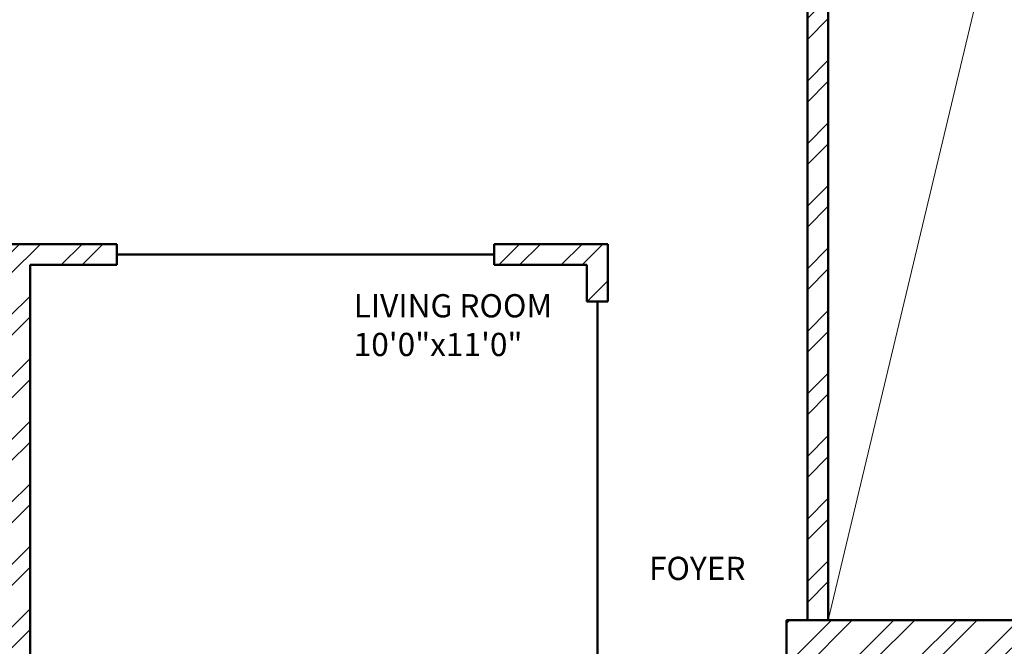
# Model space of a CAD drawing. Units: inches. Extents: x 1901 to 2863, y 888 to 2433.
# Tile 53 of 91: x 2169 to 2381, y 1867 to 2002. Entities that reach past the tile are written whole.
import ezdxf

# ---------------------------------------------------------------- set-up
doc = ezdxf.new("R2010")
doc.units = ezdxf.units.IN
for name, color, linetype, lineweight in [('A-ANNO-SYMB', 8, 'Continuous', 13), ('A-AREA-IDEN', 7, 'Continuous', 18), ('A-WALL', 7, 'Continuous', 50), ('A-WALL-PATT', 8, 'Continuous', 13)]:
    doc.layers.add(name, color=color, linetype=linetype, lineweight=lineweight)
doc.styles.get("Standard").update_dxf_attribs({"font": 'arial.ttf'})

msp = doc.modelspace()

# ---------------------------------------------------------------- hatches: boundary and pattern name
at = {"layer": 'A-WALL-PATT'}
h = msp.add_hatch(dxfattribs=at)
h.set_pattern_fill('ANSI32', color=256)
h.paths.add_polyline_path([(2192.5, 2274.13), (2141.26, 2274.13), (2141.26, 2269.63), (2192.5, 2269.63)])
h.paths.add_polyline_path([(2259.93, 2274.13), (2216.5, 2274.13), (2216.5, 2269.63), (2255.43, 2269.63), (2255.43, 2214.63), (2250.81, 2214.63), (2250.81, 2210.13), (2259.93, 2210.13), (2259.93, 2215.13), (2271.76, 2215.13), (2271.76, 2217.38), (2271.76, 2219.63), (2259.93, 2219.63)])
h.paths.add_polyline_path([(2171.43, 2269.63), (2166.93, 2269.63), (2166.93, 2219.63), (2121.24, 2219.63), (2121.24, 2215.13), (2166.93, 2215.13), (2166.93, 2083.13), (2161.81, 2083.13), (2161.81, 2078.63), (2171.43, 2078.63), (2177, 2078.63), (2177, 2080.88), (2177, 2083.13), (2171.43, 2083.13), (2171.43, 2210.13), (2230.91, 2210.13), (2230.91, 2212.38), (2230.91, 2214.63), (2171.43, 2214.63)])
h.paths.add_polyline_path([(2117.26, 2274.13), (2089.43, 2274.13), (2089.43, 2219.63), (2081.14, 2219.63), (2081.14, 2215.13), (2089.43, 2215.13), (2098, 2215.13), (2098, 2217.38), (2098, 2219.63), (2093.93, 2219.63), (2093.93, 2269.63), (2117.26, 2269.63), (2117.26, 2271.88)])
h.paths.add_polyline_path([(2343.43, 2219.63), (2329.29, 2219.63), (2329.29, 2215.13), (2338.93, 2215.13), (2338.93, 2184.74), (2343.43, 2184.74)])
h.paths.add_polyline_path([(2338.93, 2083.13), (2329.29, 2083.13), (2208.97, 2083.13), (2208.97, 2078.63), (2338.93, 2078.63)])
h.paths.add_polyline_path([(2343.43, 2136.74), (2338.93, 2136.74), (2338.93, 1872.63), (2343.43, 1872.63)])
h.paths.add_polyline_path([(2343.43, 1863.63), (2397.68, 1863.63), (2397.68, 1821.63), (2384.14, 1821.63), (2384.14, 1812.63), (2418.33, 1812.63), (2418.33, 1817.13), (2418.33, 1821.63), (2406.68, 1821.63), (2406.68, 1863.63), (2459.5, 1863.63), (2459.5, 1821.63), (2447.14, 1821.63), (2447.14, 1812.63), (2459.5, 1812.63), (2468.5, 1812.63), (2468.5, 1872.63), (2394.43, 1872.63), (2334.43, 1872.63), (2334.43, 1812.63), (2343.43, 1812.63), (2353.25, 1812.63), (2353.25, 1821.63), (2343.43, 1821.63)])
h.paths.add_polyline_path([(2510.01, 1872.63), (2468.5, 1872.63), (2468.5, 1868.13), (2510.01, 1868.13)])
h.paths.add_polyline_path([(2514.01, 1817.13), (2468.5, 1817.13), (2468.5, 1812.63), (2482.11, 1812.63), (2482.11, 1800.61), (2486.61, 1800.61), (2486.61, 1812.63), (2514.01, 1812.63)])
h.paths.add_polyline_path([(2299.25, 1814.88), (2299.25, 1817.13), (2295.93, 1817.13), (2295.93, 1854.17), (2293.68, 1854.17), (2291.43, 1854.17), (2291.43, 1817.13), (2266.11, 1817.13), (2266.11, 1812.63), (2299.25, 1812.63)])
h.paths.add_polyline_path([(2218.11, 1817.13), (2206.46, 1817.13), (2171.43, 1817.13), (2171.43, 1949.13), (2190.1, 1949.13), (2190.1, 1953.63), (2163.47, 1953.63), (2163.47, 1949.13), (2166.93, 1949.13), (2166.93, 1817.13), (2114.3, 1817.13), (2114.3, 1812.63), (2218.11, 1812.63)])
h.paths.add_polyline_path([(2029.43, 1970.92), (2024.93, 1970.92), (2024.93, 1912.72), (2029.43, 1912.72)])
h.paths.add_polyline_path([(2132.3, 1953.63), (2113.93, 1953.63), (2113.93, 1975.89), (2111.68, 1975.89), (2109.43, 1975.89), (2109.43, 1953.63), (2029.43, 1953.63), (2029.43, 1949.13), (2132.3, 1949.13)])
h.paths.add_polyline_path([(2029.43, 1853.61), (2029.31, 1853.61), (2029.31, 1853.61), (2029.43, 1853.61), (2029.43, 1864.72), (2024.93, 1864.72), (2024.93, 1812.63), (2066.3, 1812.63), (2066.3, 1814.88), (2066.3, 1817.13), (2029.43, 1817.13)])
h.paths.add_polyline_path([(2122.93, 2010.09), (2120.68, 2010.09), (2118.43, 2010.09), (2118.43, 2006.13), (2029.43, 2006.13), (2029.43, 2001.63), (2109.43, 2001.63), (2109.43, 1998.04), (2113.93, 1998.04), (2113.93, 2001.63), (2122.93, 2001.63)])
h.paths.add_polyline_path([(2029.43, 2031.38), (2024.93, 2031.38), (2024.93, 1994.92), (2027.18, 1994.92), (2029.43, 1994.92)])
h.paths.add_polyline_path([(2029.43, 2136.74), (2024.93, 2136.74), (2024.93, 2067.38), (2027.18, 2067.38), (2029.43, 2067.38)])
h.paths.add_polyline_path([(2125.62, 2083.13), (2029.43, 2083.13), (2029.43, 2078.63), (2118.43, 2078.63), (2118.43, 2030.71), (2122.93, 2030.71), (2122.93, 2078.63), (2125.62, 2078.63)])
h.paths.add_polyline_path([(2029.43, 2215.13), (2040.47, 2215.13), (2040.47, 2217.38), (2040.47, 2219.63), (2024.93, 2219.63), (2024.93, 2184.74), (2029.43, 2184.74), (2029.43, 2187.78)])
h.paths.add_polyline_path([(2686.43, 2274.13), (2659.28, 2274.13), (2659.28, 2269.63), (2681.93, 2269.63), (2681.93, 2219.63), (2676.82, 2219.63), (2676.82, 2215.13), (2681.93, 2215.13), (2697.01, 2215.13), (2697.01, 2217.38), (2697.01, 2219.63), (2686.43, 2219.63)])
h.paths.add_polyline_path([(2609.93, 2269.63), (2635.28, 2269.63), (2635.28, 2274.13), (2571.43, 2274.13), (2571.43, 2269.63), (2605.43, 2269.63), (2605.43, 2214.63), (2549.1, 2214.63), (2549.1, 2210.13), (2605.43, 2210.13), (2605.43, 2083.13), (2601.01, 2083.13), (2601.01, 2080.88), (2601.01, 2078.63), (2609.93, 2078.63), (2616.16, 2078.63), (2616.16, 2080.88), (2616.16, 2083.13), (2609.93, 2083.13), (2609.93, 2215.13), (2651.46, 2215.13), (2651.46, 2217.38), (2651.46, 2219.63), (2609.93, 2219.63)])
h.paths.add_polyline_path([(2521.43, 2269.63), (2547.43, 2269.63), (2547.43, 2271.88), (2547.43, 2274.13), (2516.93, 2274.13), (2516.93, 2219.63), (2506.41, 2219.63), (2506.41, 2215.13), (2516.93, 2215.13), (2516.93, 2210.13), (2525.4, 2210.13), (2525.4, 2212.38), (2525.4, 2214.63), (2521.43, 2214.63)])
h.paths.add_polyline_path([(2456.01, 2219.63), (2439.43, 2219.63), (2439.43, 2187.89), (2443.93, 2187.89), (2443.93, 2215.13), (2456.01, 2215.13)])
h.paths.add_polyline_path([(2752.93, 2219.63), (2739.48, 2219.63), (2739.48, 2215.13), (2748.43, 2215.13), (2748.43, 2187.89), (2752.93, 2187.89)])
h.paths.add_polyline_path([(2752.93, 2139.89), (2748.43, 2139.89), (2748.43, 2083.13), (2648.42, 2083.13), (2648.42, 2078.63), (2654.93, 2078.63), (2654.93, 2039.44), (2659.43, 2039.44), (2659.43, 2078.63), (2748.43, 2078.63), (2748.43, 2063.43), (2752.93, 2063.43)])
h.paths.add_polyline_path([(2752.93, 2010.63), (2659.43, 2010.63), (2659.43, 2015.65), (2654.93, 2015.65), (2654.93, 2010.63), (2605.43, 2010.63), (2605.43, 1920.97), (2609.93, 1920.97), (2609.93, 2006.13), (2748.43, 2006.13), (2748.43, 1982.47), (2752.93, 1982.47)])
h.paths.add_polyline_path([(2752.93, 2027.43), (2748.43, 2027.43), (2748.43, 2010.63), (2752.93, 2010.63)])
h.paths.add_polyline_path([(2748.43, 1886.13), (2609.93, 1886.13), (2609.93, 1889.72), (2605.43, 1889.72), (2605.43, 1861.26), (2609.93, 1861.26), (2609.93, 1881.63), (2748.43, 1881.63)])
h.paths.add_polyline_path([(2456.86, 2228.83), (2498.4, 2228.83), (2498.4, 2247.49), (2456.86, 2247.49)], flags=9)
h.paths.add_polyline_path([(2038.6, 2237.42), (2080.17, 2237.42), (2080.17, 2256.08), (2038.6, 2256.08)], flags=9)
h.paths.add_polyline_path([(2292.01, 1062.39), (2539.93, 1062.39), (2539.93, 1099.49), (2292.01, 1099.49)], flags=9)
h.paths.add_polyline_path([(2424.91, 1832.25), (2448.51, 1832.25), (2448.51, 1846.68), (2424.91, 1846.68)], flags=25)
h.paths.add_polyline_path([(2359.08, 1832.25), (2382.68, 1832.25), (2382.68, 1846.68), (2359.08, 1846.68)], flags=25)
h.paths.add_polyline_path([(2352.9, 1684.8), (2367.54, 1684.8), (2367.54, 1697.17), (2352.9, 1697.17)], flags=9)
h.paths.add_polyline_path([(2079.29, 1755.83), (2169.02, 1755.83), (2169.02, 1774.37), (2079.29, 1774.37)], flags=9)
h.paths.add_polyline_path([(2404.09, 1373.86), (2404.09, 1463.59), (2385.54, 1463.59), (2385.54, 1373.86)], flags=9)
h.paths.add_polyline_path([(2268.09, 2236.37), (2309.64, 2236.37), (2309.64, 2255.03), (2268.09, 2255.03)], flags=9)
h.paths.add_polyline_path([(2575.96, 1700.95), (2665.7, 1700.95), (2665.7, 1719.5), (2575.96, 1719.5)], flags=9)
h.paths.add_polyline_path([(2302.96, 1878.47), (2329.52, 1878.47), (2329.52, 1888.78), (2302.96, 1888.78)], flags=9)
h.paths.add_polyline_path([(2097.42, 2240.58), (2126.57, 2240.58), (2126.57, 2259.23), (2097.42, 2259.23)], flags=9)
h.paths.add_polyline_path([(2208.72, 2246.12), (2237.88, 2246.12), (2237.88, 2264.78), (2208.72, 2264.78)], flags=9)
h.paths.add_polyline_path([(2038.15, 1925.96), (2076.99, 1925.96), (2076.99, 1944.62), (2038.15, 1944.62)], flags=9)
h.paths.add_polyline_path([(2239.14, 1926.67), (2288.46, 1926.67), (2288.46, 1945.33), (2239.14, 1945.33)], flags=9)
h.paths.add_polyline_path([(2175.43, 2007.33), (2212.36, 2007.33), (2212.36, 2025.99), (2175.43, 2025.99)], flags=9)
h.paths.add_polyline_path([(2225.03, 2091.79), (2263.87, 2091.79), (2263.87, 2110.45), (2225.03, 2110.45)], flags=9)
h.paths.add_polyline_path([(2035.4, 2098.48), (2074.24, 2098.48), (2074.24, 2117.14), (2035.4, 2117.14)], flags=9)
h.paths.add_polyline_path([(2050.1, 2029.21), (2083.26, 2029.21), (2083.26, 2047.87), (2050.1, 2047.87)], flags=9)
h.paths.add_polyline_path([(2069.68, 1956.72), (2098.83, 1956.72), (2098.83, 1975.38), (2069.68, 1975.38)], flags=25)
h.paths.add_polyline_path([(2328.62, 1753.34), (2361.66, 1753.34), (2361.66, 1771.99), (2328.62, 1771.99)], flags=9)
h.paths.add_polyline_path([(2395.16, 2060.89), (2395.16, 2140.65), (2378.68, 2140.65), (2378.68, 2060.89)], flags=9)
h.paths.add_polyline_path([(2463.73, 2059.02), (2492.89, 2059.02), (2492.89, 2077.68), (2463.73, 2077.68)], flags=9)
h.paths.add_polyline_path([(2458.03, 2181.54), (2496.87, 2181.54), (2496.87, 2200.19), (2458.03, 2200.19)], flags=9)
h.paths.add_polyline_path([(2527.58, 2243.07), (2556.73, 2243.07), (2556.73, 2261.73), (2527.58, 2261.73)], flags=9)
h.paths.add_polyline_path([(2694.46, 2232.77), (2736.03, 2232.77), (2736.03, 2251.42), (2694.46, 2251.42)], flags=9)
h.paths.add_polyline_path([(2637.82, 2249.22), (2666.98, 2249.22), (2666.98, 2267.88), (2637.82, 2267.88)], flags=9)
h.paths.add_polyline_path([(2623.69, 2183.54), (2662.53, 2183.54), (2662.53, 2202.2), (2623.69, 2202.2)], flags=9)
h.paths.add_polyline_path([(2691.97, 2021.5), (2725.12, 2021.5), (2725.12, 2040.16), (2691.97, 2040.16)], flags=9)
h.paths.add_polyline_path([(2621.04, 1975.91), (2662.34, 1975.91), (2662.34, 1994.57), (2621.04, 1994.57)], flags=25)
h.paths.add_polyline_path([(2479.03, 1927.62), (2519.84, 1927.62), (2519.84, 1946.28), (2479.03, 1946.28)], flags=9)
h.paths.add_polyline_path([(2670.94, 1849.08), (2716.01, 1849.08), (2716.01, 1867.73), (2670.94, 1867.73)], flags=9)
h.paths.add_polyline_path([(2523.61, 1782.96), (2550.17, 1782.96), (2550.17, 1793.26), (2523.61, 1793.26)], flags=9)
h.paths.add_polyline_path([(2450.84, 1207.33), (2492.39, 1207.33), (2492.39, 1225.99), (2450.84, 1225.99)], flags=9)
h.paths.add_polyline_path([(2527.75, 1203.84), (2556.91, 1203.84), (2556.91, 1222.5), (2527.75, 1222.5)], flags=9)
h.paths.add_polyline_path([(2639.11, 1207.2), (2668.27, 1207.2), (2668.27, 1225.86), (2639.11, 1225.86)], flags=9)
h.paths.add_polyline_path([(2692.59, 1218.97), (2734.17, 1218.97), (2734.17, 1237.62), (2692.59, 1237.62)], flags=9)
h.paths.add_polyline_path([(2669.27, 1366.33), (2708.11, 1366.33), (2708.11, 1384.99), (2669.27, 1384.99)], flags=9)
h.paths.add_polyline_path([(2463.31, 1358.03), (2502.15, 1358.03), (2502.15, 1376.69), (2463.31, 1376.69)], flags=9)
h.paths.add_polyline_path([(2494.72, 1449.96), (2531.65, 1449.96), (2531.65, 1468.62), (2494.72, 1468.62)], flags=9)
h.paths.add_polyline_path([(2675.57, 1422.16), (2708.72, 1422.16), (2708.72, 1440.81), (2675.57, 1440.81)], flags=9)
h.paths.add_polyline_path([(2685.63, 1493.89), (2714.79, 1493.89), (2714.79, 1512.55), (2685.63, 1512.55)], flags=9)
h.paths.add_polyline_path([(2686.8, 1529.91), (2725.65, 1529.91), (2725.65, 1548.57), (2686.8, 1548.57)], flags=9)
h.paths.add_polyline_path([(2503.65, 1537.99), (2552.97, 1537.99), (2552.97, 1556.65), (2503.65, 1556.65)], flags=9)
h.paths.add_polyline_path([(2291.71, 1643.5), (2318.28, 1643.5), (2318.28, 1653.81), (2291.71, 1653.81)], flags=9)
h.paths.add_polyline_path([(2450.63, 1610.52), (2477.19, 1610.52), (2477.19, 1620.82), (2450.63, 1620.82)], flags=9)
h.paths.add_polyline_path([(2359.99, 1551.81), (2422.25, 1551.81), (2422.25, 1562.12), (2359.99, 1562.12)], flags=9)
h.paths.add_polyline_path([(2280.11, 1249.01), (2321.65, 1249.01), (2321.65, 1267.66), (2280.11, 1267.66)], flags=9)
h.paths.add_polyline_path([(2164.06, 1274.23), (2193.22, 1274.23), (2193.22, 1292.89), (2164.06, 1292.89)], flags=9)
h.paths.add_polyline_path([(2118.21, 1277.69), (2151.25, 1277.69), (2151.25, 1296.35), (2118.21, 1296.35)], flags=9)
h.paths.add_polyline_path([(2031.95, 1268.53), (2073.52, 1268.53), (2073.52, 1287.19), (2031.95, 1287.19)], flags=9)
h.paths.add_polyline_path([(2050.2, 1409.08), (2089.04, 1409.08), (2089.04, 1427.74), (2050.2, 1427.74)], flags=9)
h.paths.add_polyline_path([(2243.74, 1421.03), (2282.58, 1421.03), (2282.58, 1439.69), (2243.74, 1439.69)], flags=9)
h.paths.add_polyline_path([(2190.75, 1509.77), (2231.56, 1509.77), (2231.56, 1528.43), (2190.75, 1528.43)], flags=9)
h.paths.add_polyline_path([(2058.39, 1475.42), (2091.55, 1475.42), (2091.55, 1494.07), (2058.39, 1494.07)], flags=9)
h.paths.add_polyline_path([(2062.45, 1553.09), (2091.6, 1553.09), (2091.6, 1571.75), (2062.45, 1571.75)], flags=9)
h.paths.add_polyline_path([(2219.52, 1590.37), (2266.15, 1590.37), (2266.15, 1609.02), (2219.52, 1609.02)], flags=9)
h.paths.add_polyline_path([(2041.07, 1584.19), (2079.91, 1584.19), (2079.91, 1602.85), (2041.07, 1602.85)], flags=9)
h = msp.add_hatch(dxfattribs=at)
h.set_pattern_fill('ANSI32', color=256)
h.paths.add_polyline_path([(2443.93, 2139.89), (2439.43, 2139.89), (2439.43, 2069.35), (2441.68, 2069.35), (2443.93, 2069.35), (2443.93, 2078.63), (2521.93, 2078.63), (2521.93, 2075.07), (2524.18, 2075.07), (2526.43, 2075.07), (2526.43, 2078.63), (2571.75, 2078.63), (2571.75, 2080.88), (2571.75, 2083.13), (2443.93, 2083.13)])
h.paths.add_polyline_path([(2526.43, 2054.63), (2524.18, 2054.63), (2521.93, 2054.63), (2521.93, 2030.63), (2443.93, 2030.63), (2443.93, 2045.35), (2439.43, 2045.35), (2439.43, 1983.87), (2443.93, 1983.87), (2443.93, 2026.13), (2521.93, 2026.13), (2526.43, 2026.13)])
h.paths.add_polyline_path([(2443.93, 1923.87), (2439.43, 1923.87), (2439.43, 1872.63), (2443.93, 1872.63)])
h.paths.add_polyline_path([(2636.23, 1766.13), (2609.93, 1766.13), (2609.93, 1779.79), (2605.43, 1779.79), (2605.43, 1766.13), (2486.61, 1766.13), (2486.61, 1770.67), (2482.11, 1770.67), (2482.11, 1766.13), (2482.11, 1761.63), (2636.23, 1761.63), (2636.23, 1763.88)])
h.paths.add_polyline_path([(2519.54, 1663.38), (2519.54, 1665.63), (2494.93, 1665.63), (2481.83, 1665.63), (2481.83, 1663.38), (2481.83, 1661.13), (2490.43, 1661.13), (2490.43, 1640.16), (2494.93, 1640.16), (2494.93, 1661.13), (2519.54, 1661.13)])
h.paths.add_polyline_path([(2443.93, 1712.13), (2443.93, 1716.63), (2414.46, 1716.63), (2414.46, 1712.13), (2439.43, 1712.13), (2439.43, 1545.51), (2443.93, 1545.51), (2443.93, 1661.13), (2448.47, 1661.13), (2448.47, 1665.63), (2443.93, 1665.63)])
h.paths.add_polyline_path([(2343.43, 1712.13), (2365.52, 1712.13), (2365.52, 1714.38), (2365.52, 1716.63), (2333.87, 1716.63), (2333.87, 1714.38), (2333.87, 1712.13), (2338.93, 1712.13), (2338.93, 1575.63), (2338.93, 1545.51), (2343.43, 1545.51), (2343.43, 1547.51), (2343.43, 1580.13)])
h.paths.add_polyline_path([(2752.93, 1665.63), (2579.54, 1665.63), (2579.54, 1661.13), (2615.93, 1661.13), (2615.93, 1529.13), (2598.93, 1529.13), (2598.93, 1524.63), (2623.13, 1524.63), (2623.13, 1526.88), (2623.13, 1529.13), (2620.43, 1529.13), (2620.43, 1661.13), (2748.43, 1661.13), (2748.43, 1633.5), (2752.93, 1633.5)])
h.paths.add_polyline_path([(2752.93, 1419.93), (2748.43, 1419.93), (2748.43, 1400.13), (2659.43, 1400.13), (2659.43, 1444.33), (2657.18, 1444.33), (2654.93, 1444.33), (2654.93, 1400.13), (2643.65, 1400.13), (2643.65, 1395.63), (2748.43, 1395.63), (2748.43, 1364.04), (2752.93, 1364.04)])
h.paths.add_polyline_path([(2752.93, 1492.88), (2748.43, 1492.88), (2748.43, 1476.63), (2667.43, 1476.63), (2667.43, 1479.71), (2665.18, 1479.71), (2662.93, 1479.71), (2662.93, 1476.63), (2654.93, 1476.63), (2654.93, 1469.54), (2659.43, 1469.54), (2659.43, 1472.13), (2748.43, 1472.13), (2748.43, 1455.93), (2752.93, 1455.93)])
h.paths.add_polyline_path([(2752.93, 1304.04), (2748.43, 1304.04), (2748.43, 1263.63), (2738.66, 1263.63), (2738.66, 1259.13), (2752.93, 1259.13)])
h.paths.add_polyline_path([(2685.93, 1259.13), (2695.49, 1259.13), (2695.49, 1261.38), (2695.49, 1263.63), (2677.84, 1263.63), (2677.84, 1261.38), (2677.84, 1259.13), (2681.43, 1259.13), (2681.43, 1203.63), (2653.28, 1203.63), (2653.28, 1199.13), (2685.93, 1199.13), (2685.93, 1203.63)])
h.paths.add_polyline_path([(2609.43, 1395.63), (2611.85, 1395.63), (2611.85, 1400.13), (2598.89, 1400.13), (2598.89, 1397.88), (2598.89, 1395.63), (2604.93, 1395.63), (2604.93, 1268.13), (2554.73, 1268.13), (2554.73, 1265.88), (2554.73, 1263.63), (2604.93, 1263.63), (2604.93, 1203.63), (2571.31, 1203.63), (2571.31, 1199.13), (2604.93, 1199.13), (2629.28, 1199.13), (2629.28, 1201.38), (2629.28, 1203.63), (2609.43, 1203.63), (2609.43, 1258.63), (2609.43, 1259.13), (2654.8, 1259.13), (2654.8, 1263.63), (2609.43, 1263.63)])
h.paths.add_polyline_path([(2443.93, 1304.04), (2439.43, 1304.04), (2439.43, 1259.13), (2443.93, 1259.13), (2456.16, 1259.13), (2456.16, 1261.38), (2456.16, 1263.63), (2443.93, 1263.63)])
h.paths.add_polyline_path([(2525.43, 1263.63), (2531.78, 1263.63), (2531.78, 1268.13), (2520.93, 1268.13), (2520.93, 1263.63), (2511.41, 1263.63), (2511.41, 1259.13), (2520.93, 1259.13), (2520.93, 1199.13), (2547.31, 1199.13), (2547.31, 1201.38), (2547.31, 1203.63), (2525.43, 1203.63)])
h.paths.add_polyline_path([(2443.93, 1434.84), (2439.43, 1434.84), (2439.43, 1364.04), (2441.68, 1364.04), (2443.93, 1364.04)])
h.paths.add_polyline_path([(2567.13, 1400.13), (2443.93, 1400.13), (2443.93, 1395.63), (2567.13, 1395.63)])
h.paths.add_polyline_path([(2443.93, 1545.51), (2439.43, 1545.51), (2439.43, 1494.84), (2443.93, 1494.84)])
h.paths.add_polyline_path([(2494.93, 1553.35), (2492.68, 1553.35), (2490.43, 1553.35), (2490.43, 1524.63), (2494.93, 1524.63), (2525.94, 1524.63), (2525.94, 1526.88), (2525.94, 1529.13), (2494.93, 1529.13)])
h.paths.add_polyline_path([(2752.93, 1573.5), (2748.43, 1573.5), (2748.43, 1529.13), (2657.76, 1529.13), (2657.76, 1524.63), (2662.93, 1524.63), (2662.93, 1498.63), (2667.43, 1498.63), (2667.43, 1524.63), (2748.43, 1524.63), (2748.43, 1516.88), (2752.93, 1516.88)])
h.paths.add_polyline_path([(2038.6, 2237.42), (2080.17, 2237.42), (2080.17, 2256.08), (2038.6, 2256.08)], flags=9)
h.paths.add_polyline_path([(2292.01, 1062.39), (2539.93, 1062.39), (2539.93, 1099.49), (2292.01, 1099.49)], flags=9)
h.paths.add_polyline_path([(2424.91, 1832.25), (2448.51, 1832.25), (2448.51, 1846.68), (2424.91, 1846.68)], flags=9)
h.paths.add_polyline_path([(2359.08, 1832.25), (2382.68, 1832.25), (2382.68, 1846.68), (2359.08, 1846.68)], flags=9)
h.paths.add_polyline_path([(2352.9, 1684.8), (2367.54, 1684.8), (2367.54, 1697.17), (2352.9, 1697.17)], flags=9)
h.paths.add_polyline_path([(2079.29, 1755.83), (2169.02, 1755.83), (2169.02, 1774.37), (2079.29, 1774.37)], flags=9)
h.paths.add_polyline_path([(2404.09, 1373.86), (2404.09, 1463.59), (2385.54, 1463.59), (2385.54, 1373.86)], flags=9)
h.paths.add_polyline_path([(2268.09, 2236.37), (2309.64, 2236.37), (2309.64, 2255.03), (2268.09, 2255.03)], flags=9)
h.paths.add_polyline_path([(2575.96, 1700.95), (2665.7, 1700.95), (2665.7, 1719.5), (2575.96, 1719.5)], flags=9)
h.paths.add_polyline_path([(2302.96, 1878.47), (2329.52, 1878.47), (2329.52, 1888.78), (2302.96, 1888.78)], flags=9)
h.paths.add_polyline_path([(2097.42, 2240.58), (2126.57, 2240.58), (2126.57, 2259.23), (2097.42, 2259.23)], flags=9)
h.paths.add_polyline_path([(2208.72, 2246.12), (2237.88, 2246.12), (2237.88, 2264.78), (2208.72, 2264.78)], flags=9)
h.paths.add_polyline_path([(2038.15, 1925.96), (2076.99, 1925.96), (2076.99, 1944.62), (2038.15, 1944.62)], flags=9)
h.paths.add_polyline_path([(2239.14, 1926.67), (2288.46, 1926.67), (2288.46, 1945.33), (2239.14, 1945.33)], flags=9)
h.paths.add_polyline_path([(2175.43, 2007.33), (2212.36, 2007.33), (2212.36, 2025.99), (2175.43, 2025.99)], flags=9)
h.paths.add_polyline_path([(2225.03, 2091.79), (2263.87, 2091.79), (2263.87, 2110.45), (2225.03, 2110.45)], flags=9)
h.paths.add_polyline_path([(2035.4, 2098.48), (2074.24, 2098.48), (2074.24, 2117.14), (2035.4, 2117.14)], flags=9)
h.paths.add_polyline_path([(2050.1, 2029.21), (2083.26, 2029.21), (2083.26, 2047.87), (2050.1, 2047.87)], flags=9)
h.paths.add_polyline_path([(2069.68, 1956.72), (2098.83, 1956.72), (2098.83, 1975.38), (2069.68, 1975.38)], flags=9)
h.paths.add_polyline_path([(2328.62, 1753.34), (2361.66, 1753.34), (2361.66, 1771.99), (2328.62, 1771.99)], flags=9)
h.paths.add_polyline_path([(2395.16, 2060.89), (2395.16, 2140.65), (2378.68, 2140.65), (2378.68, 2060.89)], flags=9)
h.paths.add_polyline_path([(2463.73, 2059.02), (2492.89, 2059.02), (2492.89, 2077.68), (2463.73, 2077.68)], flags=9)
h.paths.add_polyline_path([(2458.03, 2181.54), (2496.87, 2181.54), (2496.87, 2200.19), (2458.03, 2200.19)], flags=9)
h.paths.add_polyline_path([(2456.86, 2228.83), (2498.4, 2228.83), (2498.4, 2247.49), (2456.86, 2247.49)], flags=9)
h.paths.add_polyline_path([(2527.58, 2243.07), (2556.73, 2243.07), (2556.73, 2261.73), (2527.58, 2261.73)], flags=9)
h.paths.add_polyline_path([(2694.46, 2232.77), (2736.03, 2232.77), (2736.03, 2251.42), (2694.46, 2251.42)], flags=9)
h.paths.add_polyline_path([(2637.82, 2249.22), (2666.98, 2249.22), (2666.98, 2267.88), (2637.82, 2267.88)], flags=9)
h.paths.add_polyline_path([(2623.69, 2183.54), (2662.53, 2183.54), (2662.53, 2202.2), (2623.69, 2202.2)], flags=9)
h.paths.add_polyline_path([(2691.97, 2021.5), (2725.12, 2021.5), (2725.12, 2040.16), (2691.97, 2040.16)], flags=9)
h.paths.add_polyline_path([(2621.04, 1975.91), (2662.34, 1975.91), (2662.34, 1994.57), (2621.04, 1994.57)], flags=9)
h.paths.add_polyline_path([(2479.03, 1927.62), (2519.84, 1927.62), (2519.84, 1946.28), (2479.03, 1946.28)], flags=9)
h.paths.add_polyline_path([(2670.94, 1849.08), (2716.01, 1849.08), (2716.01, 1867.73), (2670.94, 1867.73)], flags=9)
h.paths.add_polyline_path([(2523.61, 1782.96), (2550.17, 1782.96), (2550.17, 1793.26), (2523.61, 1793.26)], flags=9)
h.paths.add_polyline_path([(2450.84, 1207.33), (2492.39, 1207.33), (2492.39, 1225.99), (2450.84, 1225.99)], flags=9)
h.paths.add_polyline_path([(2527.75, 1203.84), (2556.91, 1203.84), (2556.91, 1222.5), (2527.75, 1222.5)], flags=9)
h.paths.add_polyline_path([(2639.11, 1207.2), (2668.27, 1207.2), (2668.27, 1225.86), (2639.11, 1225.86)], flags=9)
h.paths.add_polyline_path([(2692.59, 1218.97), (2734.17, 1218.97), (2734.17, 1237.62), (2692.59, 1237.62)], flags=9)
h.paths.add_polyline_path([(2669.27, 1366.33), (2708.11, 1366.33), (2708.11, 1384.99), (2669.27, 1384.99)], flags=25)
h.paths.add_polyline_path([(2463.31, 1358.03), (2502.15, 1358.03), (2502.15, 1376.69), (2463.31, 1376.69)], flags=9)
h.paths.add_polyline_path([(2494.72, 1449.96), (2531.65, 1449.96), (2531.65, 1468.62), (2494.72, 1468.62)], flags=9)
h.paths.add_polyline_path([(2675.57, 1422.16), (2708.72, 1422.16), (2708.72, 1440.81), (2675.57, 1440.81)], flags=25)
h.paths.add_polyline_path([(2685.63, 1493.89), (2714.79, 1493.89), (2714.79, 1512.55), (2685.63, 1512.55)], flags=9)
h.paths.add_polyline_path([(2686.8, 1529.91), (2725.65, 1529.91), (2725.65, 1548.57), (2686.8, 1548.57)], flags=25)
h.paths.add_polyline_path([(2503.65, 1537.99), (2552.97, 1537.99), (2552.97, 1556.65), (2503.65, 1556.65)], flags=9)
h.paths.add_polyline_path([(2291.71, 1643.5), (2318.28, 1643.5), (2318.28, 1653.81), (2291.71, 1653.81)], flags=9)
h.paths.add_polyline_path([(2450.63, 1610.52), (2477.19, 1610.52), (2477.19, 1620.82), (2450.63, 1620.82)], flags=9)
h.paths.add_polyline_path([(2359.99, 1551.81), (2422.25, 1551.81), (2422.25, 1562.12), (2359.99, 1562.12)], flags=9)
h.paths.add_polyline_path([(2280.11, 1249.01), (2321.65, 1249.01), (2321.65, 1267.66), (2280.11, 1267.66)], flags=9)
h.paths.add_polyline_path([(2164.06, 1274.23), (2193.22, 1274.23), (2193.22, 1292.89), (2164.06, 1292.89)], flags=9)
h.paths.add_polyline_path([(2118.21, 1277.69), (2151.25, 1277.69), (2151.25, 1296.35), (2118.21, 1296.35)], flags=9)
h.paths.add_polyline_path([(2031.95, 1268.53), (2073.52, 1268.53), (2073.52, 1287.19), (2031.95, 1287.19)], flags=9)
h.paths.add_polyline_path([(2050.2, 1409.08), (2089.04, 1409.08), (2089.04, 1427.74), (2050.2, 1427.74)], flags=9)
h.paths.add_polyline_path([(2243.74, 1421.03), (2282.58, 1421.03), (2282.58, 1439.69), (2243.74, 1439.69)], flags=9)
h.paths.add_polyline_path([(2190.75, 1509.77), (2231.56, 1509.77), (2231.56, 1528.43), (2190.75, 1528.43)], flags=9)
h.paths.add_polyline_path([(2058.39, 1475.42), (2091.55, 1475.42), (2091.55, 1494.07), (2058.39, 1494.07)], flags=9)
h.paths.add_polyline_path([(2062.45, 1553.09), (2091.6, 1553.09), (2091.6, 1571.75), (2062.45, 1571.75)], flags=9)
h.paths.add_polyline_path([(2219.52, 1590.37), (2266.15, 1590.37), (2266.15, 1609.02), (2219.52, 1609.02)], flags=9)
h.paths.add_polyline_path([(2041.07, 1584.19), (2079.91, 1584.19), (2079.91, 1602.85), (2041.07, 1602.85)], flags=9)
h = msp.add_hatch(dxfattribs=at)
h.set_pattern_fill('ANSI32', color=256)
h.paths.add_polyline_path([(2182.93, 1716.63), (2024.93, 1716.63), (2024.93, 1681.7), (2029.33, 1681.7), (2029.33, 1712.13), (2154.33, 1712.13), (2154.33, 1580.13), (2148.52, 1580.13), (2148.52, 1577.88), (2148.52, 1575.63), (2194.93, 1575.63), (2194.93, 1580.13), (2158.83, 1580.13), (2158.83, 1712.13), (2182.93, 1712.13)])
h.paths.add_polyline_path([(2301.07, 1716.63), (2242.93, 1716.63), (2242.93, 1712.13), (2283.83, 1712.13), (2283.83, 1685.54), (2288.33, 1685.54), (2288.33, 1712.13), (2301.07, 1712.13)])
h.paths.add_polyline_path([(2288.33, 1600.41), (2286.08, 1600.41), (2283.83, 1600.41), (2283.83, 1580.13), (2270.6, 1580.13), (2270.6, 1575.63), (2288.33, 1575.63)])
h.paths.add_polyline_path([(2295.93, 1953.63), (2271.45, 1953.63), (2271.45, 1949.13), (2291.43, 1949.13), (2291.43, 1941.24), (2295.93, 1941.24)])
h.paths.add_polyline_path([(2098.38, 1244.13), (2082.33, 1244.13), (2082.33, 1302.13), (2086.52, 1302.13), (2086.52, 1306.63), (2067.46, 1306.63), (2067.46, 1302.13), (2077.83, 1302.13), (2077.83, 1239.63), (2098.38, 1239.63), (2098.38, 1241.88)])
h.paths.add_polyline_path([(2217.31, 1306.63), (2158.83, 1306.63), (2158.83, 1451.63), (2162.72, 1451.63), (2162.72, 1453.88), (2162.72, 1456.13), (2154.33, 1456.13), (2154.33, 1443.13), (2151.91, 1443.13), (2151.91, 1438.63), (2154.33, 1438.63), (2154.33, 1306.63), (2109.31, 1306.63), (2109.31, 1304.38), (2109.31, 1302.13), (2154.33, 1302.13), (2154.33, 1244.13), (2122.38, 1244.13), (2122.38, 1239.63), (2154.33, 1239.63), (2154.33, 1223.63), (2163.33, 1223.63), (2181.01, 1223.63), (2181.01, 1225.88), (2181.01, 1228.13), (2163.33, 1228.13), (2163.33, 1258.22), (2158.83, 1258.22), (2158.83, 1302.13), (2217.31, 1302.13)])
h.paths.add_polyline_path([(2259.99, 1306.63), (2238.3, 1306.63), (2238.3, 1304.38), (2238.3, 1302.13), (2242.83, 1302.13), (2242.83, 1228.13), (2205.01, 1228.13), (2205.01, 1223.63), (2247.33, 1223.63), (2247.33, 1302.13), (2259.99, 1302.13), (2259.99, 1304.38)])
h.paths.add_polyline_path([(2343.43, 1361.7), (2338.93, 1361.7), (2338.93, 1306.63), (2322.38, 1306.63), (2322.38, 1302.13), (2343.43, 1302.13)])
h.paths.add_polyline_path([(2343.43, 1470.4), (2338.93, 1470.4), (2338.93, 1456.13), (2193.73, 1456.13), (2193.73, 1453.88), (2193.73, 1451.63), (2338.93, 1451.63), (2338.93, 1421.7), (2343.43, 1421.7)])
h.paths.add_polyline_path([(2343.43, 1545.51), (2338.93, 1545.51), (2338.93, 1530.4), (2343.43, 1530.4)])
h.paths.add_polyline_path([(2029.33, 1466.83), (2024.93, 1466.83), (2024.93, 1409.82), (2029.33, 1409.82)])
h.paths.add_polyline_path([(2122.84, 1440.88), (2122.84, 1443.13), (2121.83, 1443.13), (2121.83, 1498.18), (2119.58, 1498.18), (2117.33, 1498.18), (2117.33, 1443.13), (2029.33, 1443.13), (2029.33, 1438.63), (2122.84, 1438.63)])
h.paths.add_polyline_path([(2029.33, 1543.05), (2024.93, 1543.05), (2024.93, 1502.83), (2029.33, 1502.83)])
h.paths.add_polyline_path([(2029.33, 1621.7), (2024.93, 1621.7), (2024.93, 1567.05), (2027.13, 1567.05), (2029.33, 1567.05), (2029.33, 1575.63), (2109.33, 1575.63), (2109.33, 1554.71), (2113.83, 1554.71), (2113.83, 1575.63), (2115.8, 1575.63), (2115.8, 1577.88), (2115.8, 1580.13), (2029.33, 1580.13)])
h.paths.add_polyline_path([(2121.83, 1527.63), (2117.33, 1527.63), (2113.83, 1527.63), (2113.83, 1533.01), (2111.58, 1533.01), (2109.33, 1533.01), (2109.33, 1527.63), (2029.33, 1527.63), (2029.33, 1523.13), (2117.33, 1523.13), (2117.33, 1519.43), (2121.83, 1519.43)])
h.paths.add_polyline_path([(2029.33, 1349.82), (2024.93, 1349.82), (2024.93, 1302.13), (2036.28, 1302.13), (2036.28, 1306.63), (2029.33, 1306.63)])

# ---------------------------------------------------------------- linework, layer by layer
at = {"layer": 'A-ANNO-SYMB'}
msp.add_line((2343.43, 1872.63), (2439.43, 2274.13), dxfattribs=at)
at = {"layer": 'A-WALL'}
for p, q in [((2343.43, 2219.63), (2343.43, 1872.63)), ((2338.93, 2215.13), (2338.93, 1872.63)), ((2163.47, 1953.63), (2190.1, 1953.63)), ((2190.1, 1953.63), (2190.1, 1949.13)), ((2271.45, 1953.63), (2271.45, 1949.13)), ((2271.45, 1953.63), (2295.93, 1953.63)), ((2295.93, 1953.63), (2295.93, 1941.24)), ((2190.1, 1951.38), (2271.45, 1951.38)), ((2171.43, 1949.13), (2171.43, 1817.13)), ((2171.43, 1949.13), (2190.1, 1949.13)), ((2271.45, 1949.13), (2291.43, 1949.13)), ((2291.43, 1949.13), (2291.43, 1941.24)), ((2291.43, 1941.24), (2295.93, 1941.24)), ((2293.68, 1854.17), (2293.68, 1941.24)), ((2334.43, 1812.63), (2334.43, 1872.63)), ((2334.43, 1872.63), (2394.43, 1872.63))]:
    msp.add_line(p, q, dxfattribs=at)

# ---------------------------------------------------------------- texts
at = {"layer": 'A-AREA-IDEN', "char_height": 5, "attachment_point": 1}
for s, width, insert in [('LIVING ROOM\\P10\'0"x11\'0"', 151.4821, (2241.15, 1942.84)), ('FOYER', 65.8856, (2304.79, 1886.29))]:
    msp.add_mtext_dynamic_manual_height_columns(s, width=width, gutter_width=12.5, heights=[0], dxfattribs=dict(at, insert=insert))

doc.saveas('drawing.dxf')
